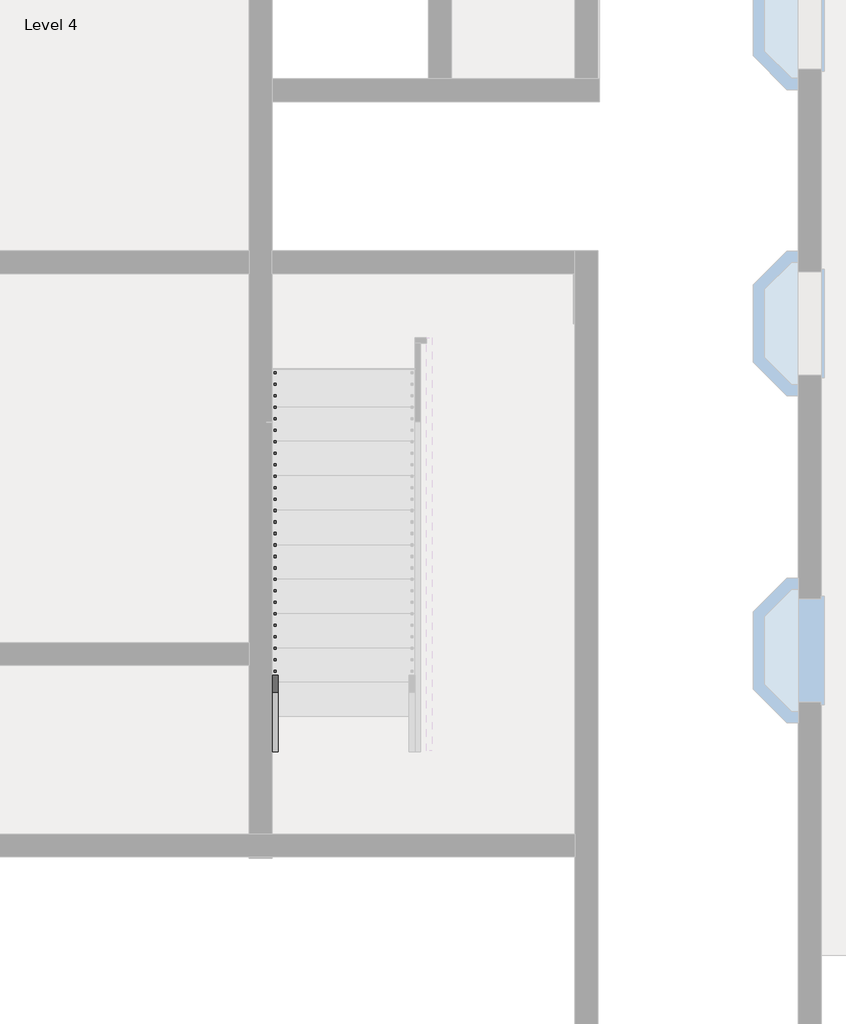
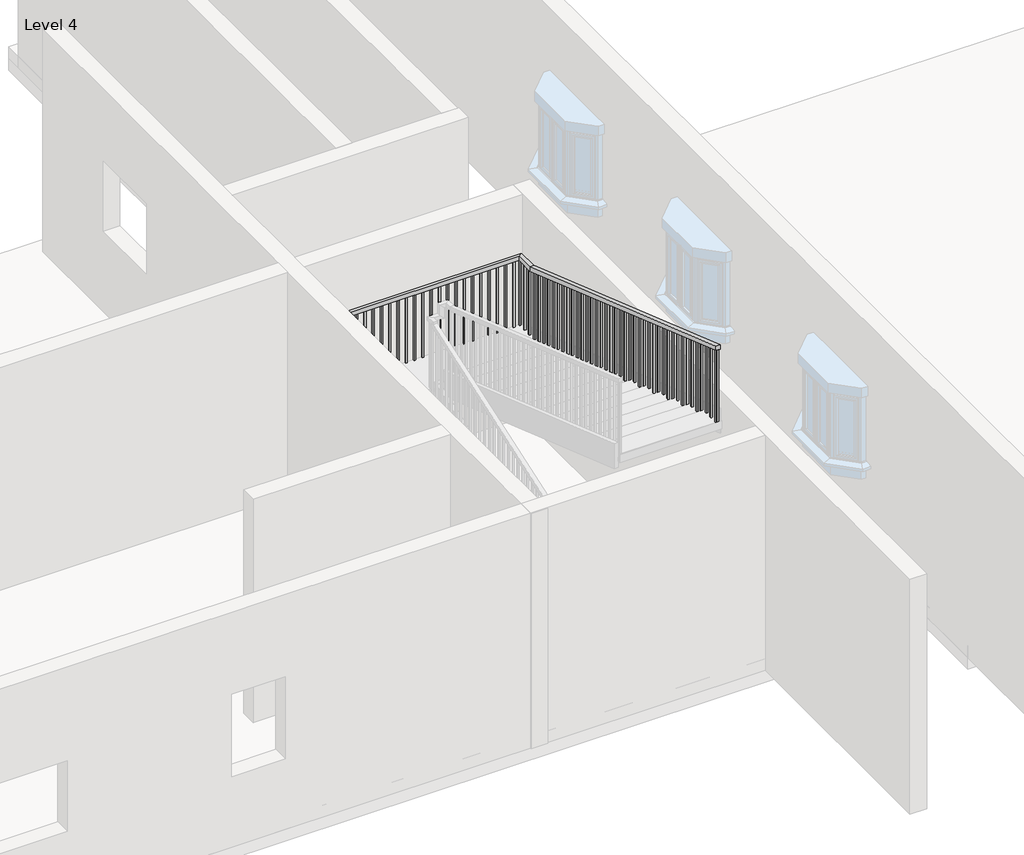
# One storey, part 8 of 14: 1 railing.
"""IFC4 building model written with IfcOpenShell, lengths in millimetres."""

from ifc_helpers import new_model, si_unit, frame, origin, place, context, project, spatial, polyline, outline, extrude, faceted_brep, element, save

model = new_model("IFC4")

# Units and contexts
model_context = context("Model", 3, world=origin())
ifc_project = project(units=[si_unit("LENGTHUNIT", "METRE", prefix="MILLI")], contexts=[model_context])

# Site, building, storey
site = spatial("IfcSite", under=ifc_project)
building = spatial("IfcBuilding", under=site)
storey = spatial("IfcBuildingStorey", under=building, Name="Level 4", Elevation=9144.0)

# Railing
placement = place(None, origin())
element("IfcRailing", 1, ObjectType="Handrail - Rectangular", at=placement, inside=storey, context=model_context, shape_type="SolidModel", body=[
    faceted_brep([(-3857.687215, -9955.5916506, 10163.9076923), (-3857.687215, -9955.5916506, 10110.1602476), (-3806.887215, -9955.5916506, 10110.1602476), (-3806.887215, -9955.5916506, 10163.9076923), (-3857.687215, -6291.6416506, 11430.0), (-3857.687215, -6283.1120276, 11379.2), (-3806.887215, -6283.1120276, 11379.2), (-3806.887215, -6291.6416506, 11430.0), (-3857.687215, -5713.7916506, 11430.0), (-3857.687215, -5713.7916506, 11379.2), (-3806.887215, -5764.5916506, 11379.2), (-3806.887215, -5764.5916506, 11430.0), (-1190.687215, -5713.7916506, 11430.0), (-1190.687215, -5713.7916506, 11379.2), (-1241.487215, -5764.5916506, 11379.2), (-1241.487215, -5764.5916506, 11430.0), (-1190.687215, -5986.8416506, 11430.0), (-1190.687215, -5995.3852679, 11379.2), (-1241.487215, -5995.3852679, 11379.2), (-1241.487215, -5986.8416506, 11430.0), (-1190.687215, -9949.2416506, 12801.6), (-1241.487215, -9949.2416506, 12801.6), (-1241.487215, -9949.2416506, 12747.842594), (-1190.687215, -9949.2416506, 12747.842594)], [[[0, 1, 2, 3]], [[1, 0, 4, 5]], [[2, 1, 5, 6]], [[3, 2, 6, 7]], [[0, 3, 7, 4]], [[5, 4, 8, 9]], [[6, 5, 9, 10]], [[7, 6, 10, 11]], [[4, 7, 11, 8]], [[9, 8, 12, 13]], [[10, 9, 13, 14]], [[11, 10, 14, 15]], [[8, 11, 15, 12]], [[13, 12, 16, 17]], [[14, 13, 17, 18]], [[15, 14, 18, 19]], [[12, 15, 19, 16]], [[20, 21, 22, 23]], [[17, 16, 20, 23]], [[18, 17, 23, 22]], [[19, 18, 22, 21]], [[16, 19, 21, 20]]]),
    extrude(outline(polyline([(-9895.2666506, 12729.1589402), (-9895.2666506, 11781.6923077), (-9914.3166506, 11781.6923077), (-9914.3166506, 12735.7531709), (-9895.2666506, 12729.1589402)])), frame((-1225.612215, 0.0, 0.0), z_axis=(1.0, 0.0, 0.0), x_axis=(0.0, 1.0, 0.0)), (0.0, 0.0, 1.0), 19.05),
    extrude(outline(polyline([(-9793.6666506, 12693.9897094), (-9793.6666506, 11781.6923077), (-9812.7166506, 11781.6923077), (-9812.7166506, 12700.5839402), (-9793.6666506, 12693.9897094)])), frame((-1225.612215, 0.0, 0.0), z_axis=(1.0, 0.0, 0.0), x_axis=(0.0, 1.0, 0.0)), (0.0, 0.0, 1.0), 19.05),
    extrude(outline(polyline([(-9692.0666506, 12658.8204786), (-9692.0666506, 11781.6923077), (-9711.1166506, 11781.6923077), (-9711.1166506, 12665.4147094), (-9692.0666506, 12658.8204786)])), frame((-1225.612215, 0.0, 0.0), z_axis=(1.0, 0.0, 0.0), x_axis=(0.0, 1.0, 0.0)), (0.0, 0.0, 1.0), 19.05),
    extrude(outline(polyline([(-9590.4666506, 12623.6512479), (-9590.4666506, 11676.1846154), (-9609.5166506, 11676.1846154), (-9609.5166506, 12630.2454786), (-9590.4666506, 12623.6512479)])), frame((-1225.612215, 0.0, 0.0), z_axis=(1.0, 0.0, 0.0), x_axis=(0.0, 1.0, 0.0)), (0.0, 0.0, 1.0), 19.05),
    extrude(outline(polyline([(-9488.8666506, 12588.4820171), (-9488.8666506, 11676.1846154), (-9507.9166506, 11676.1846154), (-9507.9166506, 12595.0762479), (-9488.8666506, 12588.4820171)])), frame((-1225.612215, 0.0, 0.0), z_axis=(1.0, 0.0, 0.0), x_axis=(0.0, 1.0, 0.0)), (0.0, 0.0, 1.0), 19.05),
    extrude(outline(polyline([(-9387.2666506, 12553.3127863), (-9387.2666506, 11676.1846154), (-9406.3166506, 11676.1846154), (-9406.3166506, 12559.9070171), (-9387.2666506, 12553.3127863)])), frame((-1225.612215, 0.0, 0.0), z_axis=(1.0, 0.0, 0.0), x_axis=(0.0, 1.0, 0.0)), (0.0, 0.0, 1.0), 19.05),
    extrude(outline(polyline([(-9285.6666506, 12518.1435556), (-9285.6666506, 11570.6769231), (-9304.7166506, 11570.6769231), (-9304.7166506, 12524.7377863), (-9285.6666506, 12518.1435556)])), frame((-1225.612215, 0.0, 0.0), z_axis=(1.0, 0.0, 0.0), x_axis=(0.0, 1.0, 0.0)), (0.0, 0.0, 1.0), 19.05),
    extrude(outline(polyline([(-9184.0666506, 12482.9743248), (-9184.0666506, 11570.6769231), (-9203.1166506, 11570.6769231), (-9203.1166506, 12489.5685556), (-9184.0666506, 12482.9743248)])), frame((-1225.612215, 0.0, 0.0), z_axis=(1.0, 0.0, 0.0), x_axis=(0.0, 1.0, 0.0)), (0.0, 0.0, 1.0), 19.05),
    extrude(outline(polyline([(-9082.4666506, 12447.805094), (-9082.4666506, 11570.6769231), (-9101.5166506, 11570.6769231), (-9101.5166506, 12454.3993248), (-9082.4666506, 12447.805094)])), frame((-1225.612215, 0.0, 0.0), z_axis=(1.0, 0.0, 0.0), x_axis=(0.0, 1.0, 0.0)), (0.0, 0.0, 1.0), 19.05),
    extrude(outline(polyline([(-8980.8666506, 12412.6358632), (-8980.8666506, 11465.1692308), (-8999.9166506, 11465.1692308), (-8999.9166506, 12419.230094), (-8980.8666506, 12412.6358632)])), frame((-1225.612215, 0.0, 0.0), z_axis=(1.0, 0.0, 0.0), x_axis=(0.0, 1.0, 0.0)), (0.0, 0.0, 1.0), 19.05),
    extrude(outline(polyline([(-8879.2666506, 12377.4666325), (-8879.2666506, 11465.1692308), (-8898.3166506, 11465.1692308), (-8898.3166506, 12384.0608632), (-8879.2666506, 12377.4666325)])), frame((-1225.612215, 0.0, 0.0), z_axis=(1.0, 0.0, 0.0), x_axis=(0.0, 1.0, 0.0)), (0.0, 0.0, 1.0), 19.05),
    extrude(outline(polyline([(-8777.6666506, 12342.2974017), (-8777.6666506, 11465.1692308), (-8796.7166506, 11465.1692308), (-8796.7166506, 12348.8916325), (-8777.6666506, 12342.2974017)])), frame((-1225.612215, 0.0, 0.0), z_axis=(1.0, 0.0, 0.0), x_axis=(0.0, 1.0, 0.0)), (0.0, 0.0, 1.0), 19.05),
    extrude(outline(polyline([(-8676.0666506, 12307.1281709), (-8676.0666506, 11359.6615385), (-8695.1166506, 11359.6615385), (-8695.1166506, 12313.7224017), (-8676.0666506, 12307.1281709)])), frame((-1225.612215, 0.0, 0.0), z_axis=(1.0, 0.0, 0.0), x_axis=(0.0, 1.0, 0.0)), (0.0, 0.0, 1.0), 19.05),
    extrude(outline(polyline([(-8574.4666506, 12271.9589402), (-8574.4666506, 11359.6615385), (-8593.5166506, 11359.6615385), (-8593.5166506, 12278.5531709), (-8574.4666506, 12271.9589402)])), frame((-1225.612215, 0.0, 0.0), z_axis=(1.0, 0.0, 0.0), x_axis=(0.0, 1.0, 0.0)), (0.0, 0.0, 1.0), 19.05),
    extrude(outline(polyline([(-8472.8666506, 12236.7897094), (-8472.8666506, 11359.6615385), (-8491.9166506, 11359.6615385), (-8491.9166506, 12243.3839402), (-8472.8666506, 12236.7897094)])), frame((-1225.612215, 0.0, 0.0), z_axis=(1.0, 0.0, 0.0), x_axis=(0.0, 1.0, 0.0)), (0.0, 0.0, 1.0), 19.05),
    extrude(outline(polyline([(-8371.2666506, 12201.6204786), (-8371.2666506, 11254.1538462), (-8390.3166506, 11254.1538462), (-8390.3166506, 12208.2147094), (-8371.2666506, 12201.6204786)])), frame((-1225.612215, 0.0, 0.0), z_axis=(1.0, 0.0, 0.0), x_axis=(0.0, 1.0, 0.0)), (0.0, 0.0, 1.0), 19.05),
    extrude(outline(polyline([(-8269.6666506, 12166.4512479), (-8269.6666506, 11254.1538462), (-8288.7166506, 11254.1538462), (-8288.7166506, 12173.0454786), (-8269.6666506, 12166.4512479)])), frame((-1225.612215, 0.0, 0.0), z_axis=(1.0, 0.0, 0.0), x_axis=(0.0, 1.0, 0.0)), (0.0, 0.0, 1.0), 19.05),
    extrude(outline(polyline([(-8168.0666506, 12131.2820171), (-8168.0666506, 11254.1538462), (-8187.1166506, 11254.1538462), (-8187.1166506, 12137.8762479), (-8168.0666506, 12131.2820171)])), frame((-1225.612215, 0.0, 0.0), z_axis=(1.0, 0.0, 0.0), x_axis=(0.0, 1.0, 0.0)), (0.0, 0.0, 1.0), 19.05),
    extrude(outline(polyline([(-8066.4666506, 12096.1127863), (-8066.4666506, 11148.6461538), (-8085.5166506, 11148.6461538), (-8085.5166506, 12102.7070171), (-8066.4666506, 12096.1127863)])), frame((-1225.612215, 0.0, 0.0), z_axis=(1.0, 0.0, 0.0), x_axis=(0.0, 1.0, 0.0)), (0.0, 0.0, 1.0), 19.05),
    extrude(outline(polyline([(-7964.8666506, 12060.9435556), (-7964.8666506, 11148.6461538), (-7983.9166506, 11148.6461538), (-7983.9166506, 12067.5377863), (-7964.8666506, 12060.9435556)])), frame((-1225.612215, 0.0, 0.0), z_axis=(1.0, 0.0, 0.0), x_axis=(0.0, 1.0, 0.0)), (0.0, 0.0, 1.0), 19.05),
    extrude(outline(polyline([(-7863.2666506, 12025.7743248), (-7863.2666506, 11148.6461538), (-7882.3166506, 11148.6461538), (-7882.3166506, 12032.3685556), (-7863.2666506, 12025.7743248)])), frame((-1225.612215, 0.0, 0.0), z_axis=(1.0, 0.0, 0.0), x_axis=(0.0, 1.0, 0.0)), (0.0, 0.0, 1.0), 19.05),
    extrude(outline(polyline([(-7761.6666506, 11990.605094), (-7761.6666506, 11043.1384615), (-7780.7166506, 11043.1384615), (-7780.7166506, 11997.1993248), (-7761.6666506, 11990.605094)])), frame((-1225.612215, 0.0, 0.0), z_axis=(1.0, 0.0, 0.0), x_axis=(0.0, 1.0, 0.0)), (0.0, 0.0, 1.0), 19.05),
    extrude(outline(polyline([(-7660.0666506, 11955.4358632), (-7660.0666506, 11043.1384615), (-7679.1166506, 11043.1384615), (-7679.1166506, 11962.030094), (-7660.0666506, 11955.4358632)])), frame((-1225.612215, 0.0, 0.0), z_axis=(1.0, 0.0, 0.0), x_axis=(0.0, 1.0, 0.0)), (0.0, 0.0, 1.0), 19.05),
    extrude(outline(polyline([(-7558.4666506, 11920.2666325), (-7558.4666506, 11043.1384615), (-7577.5166506, 11043.1384615), (-7577.5166506, 11926.8608632), (-7558.4666506, 11920.2666325)])), frame((-1225.612215, 0.0, 0.0), z_axis=(1.0, 0.0, 0.0), x_axis=(0.0, 1.0, 0.0)), (0.0, 0.0, 1.0), 19.05),
    extrude(outline(polyline([(-7456.8666506, 11885.0974017), (-7456.8666506, 10937.6307692), (-7475.9166506, 10937.6307692), (-7475.9166506, 11891.6916325), (-7456.8666506, 11885.0974017)])), frame((-1225.612215, 0.0, 0.0), z_axis=(1.0, 0.0, 0.0), x_axis=(0.0, 1.0, 0.0)), (0.0, 0.0, 1.0), 19.05),
    extrude(outline(polyline([(-7355.2666506, 11849.9281709), (-7355.2666506, 10937.6307692), (-7374.3166506, 10937.6307692), (-7374.3166506, 11856.5224017), (-7355.2666506, 11849.9281709)])), frame((-1225.612215, 0.0, 0.0), z_axis=(1.0, 0.0, 0.0), x_axis=(0.0, 1.0, 0.0)), (0.0, 0.0, 1.0), 19.05),
    extrude(outline(polyline([(-7253.6666506, 11814.7589402), (-7253.6666506, 10937.6307692), (-7272.7166506, 10937.6307692), (-7272.7166506, 11821.3531709), (-7253.6666506, 11814.7589402)])), frame((-1225.612215, 0.0, 0.0), z_axis=(1.0, 0.0, 0.0), x_axis=(0.0, 1.0, 0.0)), (0.0, 0.0, 1.0), 19.05),
    extrude(outline(polyline([(-7152.0666506, 11779.5897094), (-7152.0666506, 10832.1230769), (-7171.1166506, 10832.1230769), (-7171.1166506, 11786.1839402), (-7152.0666506, 11779.5897094)])), frame((-1225.612215, 0.0, 0.0), z_axis=(1.0, 0.0, 0.0), x_axis=(0.0, 1.0, 0.0)), (0.0, 0.0, 1.0), 19.05),
    extrude(outline(polyline([(-7050.4666506, 11744.4204786), (-7050.4666506, 10832.1230769), (-7069.5166506, 10832.1230769), (-7069.5166506, 11751.0147094), (-7050.4666506, 11744.4204786)])), frame((-1225.612215, 0.0, 0.0), z_axis=(1.0, 0.0, 0.0), x_axis=(0.0, 1.0, 0.0)), (0.0, 0.0, 1.0), 19.05),
    extrude(outline(polyline([(-6948.8666506, 11709.2512479), (-6948.8666506, 10832.1230769), (-6967.9166506, 10832.1230769), (-6967.9166506, 11715.8454786), (-6948.8666506, 11709.2512479)])), frame((-1225.612215, 0.0, 0.0), z_axis=(1.0, 0.0, 0.0), x_axis=(0.0, 1.0, 0.0)), (0.0, 0.0, 1.0), 19.05),
    extrude(outline(polyline([(-6847.2666506, 11674.0820171), (-6847.2666506, 10726.6153846), (-6866.3166506, 10726.6153846), (-6866.3166506, 11680.6762479), (-6847.2666506, 11674.0820171)])), frame((-1225.612215, 0.0, 0.0), z_axis=(1.0, 0.0, 0.0), x_axis=(0.0, 1.0, 0.0)), (0.0, 0.0, 1.0), 19.05),
    extrude(outline(polyline([(-6745.6666506, 11638.9127863), (-6745.6666506, 10726.6153846), (-6764.7166506, 10726.6153846), (-6764.7166506, 11645.5070171), (-6745.6666506, 11638.9127863)])), frame((-1225.612215, 0.0, 0.0), z_axis=(1.0, 0.0, 0.0), x_axis=(0.0, 1.0, 0.0)), (0.0, 0.0, 1.0), 19.05),
    extrude(outline(polyline([(-6644.0666506, 11603.7435556), (-6644.0666506, 10726.6153846), (-6663.1166506, 10726.6153846), (-6663.1166506, 11610.3377863), (-6644.0666506, 11603.7435556)])), frame((-1225.612215, 0.0, 0.0), z_axis=(1.0, 0.0, 0.0), x_axis=(0.0, 1.0, 0.0)), (0.0, 0.0, 1.0), 19.05),
    extrude(outline(polyline([(-6542.4666506, 11568.5743248), (-6542.4666506, 10621.1076923), (-6561.5166506, 10621.1076923), (-6561.5166506, 11575.1685556), (-6542.4666506, 11568.5743248)])), frame((-1225.612215, 0.0, 0.0), z_axis=(1.0, 0.0, 0.0), x_axis=(0.0, 1.0, 0.0)), (0.0, 0.0, 1.0), 19.05),
    extrude(outline(polyline([(-6440.8666506, 11533.405094), (-6440.8666506, 10621.1076923), (-6459.9166506, 10621.1076923), (-6459.9166506, 11539.9993248), (-6440.8666506, 11533.405094)])), frame((-1225.612215, 0.0, 0.0), z_axis=(1.0, 0.0, 0.0), x_axis=(0.0, 1.0, 0.0)), (0.0, 0.0, 1.0), 19.05),
    extrude(outline(polyline([(-6339.2666506, 11498.2358632), (-6339.2666506, 10621.1076923), (-6358.3166506, 10621.1076923), (-6358.3166506, 11504.830094), (-6339.2666506, 11498.2358632)])), frame((-1225.612215, 0.0, 0.0), z_axis=(1.0, 0.0, 0.0), x_axis=(0.0, 1.0, 0.0)), (0.0, 0.0, 1.0), 19.05),
    extrude(outline(polyline([(-6237.6666506, 11463.0666325), (-6237.6666506, 10515.6), (-6256.7166506, 10515.6), (-6256.7166506, 11469.6608632), (-6237.6666506, 11463.0666325)])), frame((-1225.612215, 0.0, 0.0), z_axis=(1.0, 0.0, 0.0), x_axis=(0.0, 1.0, 0.0)), (0.0, 0.0, 1.0), 19.05),
    extrude(outline(polyline([(-6136.0666506, 11427.8974017), (-6136.0666506, 10515.6), (-6155.1166506, 10515.6), (-6155.1166506, 11434.4916325), (-6136.0666506, 11427.8974017)])), frame((-1225.612215, 0.0, 0.0), z_axis=(1.0, 0.0, 0.0), x_axis=(0.0, 1.0, 0.0)), (0.0, 0.0, 1.0), 19.05),
    extrude(outline(polyline([(-6034.4666506, 11392.7281709), (-6034.4666506, 10515.6), (-6053.5166506, 10515.6), (-6053.5166506, 11399.3224017), (-6034.4666506, 11392.7281709)])), frame((-1225.612215, 0.0, 0.0), z_axis=(1.0, 0.0, 0.0), x_axis=(0.0, 1.0, 0.0)), (0.0, 0.0, 1.0), 19.05),
    extrude(outline(polyline([(-1206.562215, -5932.8666506), (-1206.562215, -5951.9166506), (-1225.612215, -5951.9166506), (-1225.612215, -5932.8666506), (-1206.562215, -5932.8666506)])), frame((0.0, 0.0, 10515.6), z_axis=(0.0, 0.0, 1.0), x_axis=(1.0, 0.0, 0.0)), (0.0, 0.0, 1.0), 863.6),
    extrude(outline(polyline([(-1206.562215, -5831.2666506), (-1206.562215, -5850.3166506), (-1225.612215, -5850.3166506), (-1225.612215, -5831.2666506), (-1206.562215, -5831.2666506)])), frame((0.0, 0.0, 10515.6), z_axis=(0.0, 0.0, 1.0), x_axis=(1.0, 0.0, 0.0)), (0.0, 0.0, 1.0), 863.6),
    extrude(outline(polyline([(-1301.812215, -5729.6666506), (-1282.762215, -5729.6666506), (-1282.762215, -5748.7166506), (-1301.812215, -5748.7166506), (-1301.812215, -5729.6666506)])), frame((0.0, 0.0, 10515.6), z_axis=(0.0, 0.0, 1.0), x_axis=(1.0, 0.0, 0.0)), (0.0, 0.0, 1.0), 863.6),
    extrude(outline(polyline([(-1403.412215, -5729.6666506), (-1384.362215, -5729.6666506), (-1384.362215, -5748.7166506), (-1403.412215, -5748.7166506), (-1403.412215, -5729.6666506)])), frame((0.0, 0.0, 10515.6), z_axis=(0.0, 0.0, 1.0), x_axis=(1.0, 0.0, 0.0)), (0.0, 0.0, 1.0), 863.6),
    extrude(outline(polyline([(-1505.012215, -5729.6666506), (-1485.962215, -5729.6666506), (-1485.962215, -5748.7166506), (-1505.012215, -5748.7166506), (-1505.012215, -5729.6666506)])), frame((0.0, 0.0, 10515.6), z_axis=(0.0, 0.0, 1.0), x_axis=(1.0, 0.0, 0.0)), (0.0, 0.0, 1.0), 863.6),
    extrude(outline(polyline([(-1606.612215, -5729.6666506), (-1587.562215, -5729.6666506), (-1587.562215, -5748.7166506), (-1606.612215, -5748.7166506), (-1606.612215, -5729.6666506)])), frame((0.0, 0.0, 10515.6), z_axis=(0.0, 0.0, 1.0), x_axis=(1.0, 0.0, 0.0)), (0.0, 0.0, 1.0), 863.6),
    extrude(outline(polyline([(-1708.212215, -5729.6666506), (-1689.162215, -5729.6666506), (-1689.162215, -5748.7166506), (-1708.212215, -5748.7166506), (-1708.212215, -5729.6666506)])), frame((0.0, 0.0, 10515.6), z_axis=(0.0, 0.0, 1.0), x_axis=(1.0, 0.0, 0.0)), (0.0, 0.0, 1.0), 863.6),
    extrude(outline(polyline([(-1809.812215, -5729.6666506), (-1790.762215, -5729.6666506), (-1790.762215, -5748.7166506), (-1809.812215, -5748.7166506), (-1809.812215, -5729.6666506)])), frame((0.0, 0.0, 10515.6), z_axis=(0.0, 0.0, 1.0), x_axis=(1.0, 0.0, 0.0)), (0.0, 0.0, 1.0), 863.6),
    extrude(outline(polyline([(-1911.412215, -5729.6666506), (-1892.362215, -5729.6666506), (-1892.362215, -5748.7166506), (-1911.412215, -5748.7166506), (-1911.412215, -5729.6666506)])), frame((0.0, 0.0, 10515.6), z_axis=(0.0, 0.0, 1.0), x_axis=(1.0, 0.0, 0.0)), (0.0, 0.0, 1.0), 863.6),
    extrude(outline(polyline([(-2013.012215, -5729.6666506), (-1993.962215, -5729.6666506), (-1993.962215, -5748.7166506), (-2013.012215, -5748.7166506), (-2013.012215, -5729.6666506)])), frame((0.0, 0.0, 10515.6), z_axis=(0.0, 0.0, 1.0), x_axis=(1.0, 0.0, 0.0)), (0.0, 0.0, 1.0), 863.6),
    extrude(outline(polyline([(-2114.612215, -5729.6666506), (-2095.562215, -5729.6666506), (-2095.562215, -5748.7166506), (-2114.612215, -5748.7166506), (-2114.612215, -5729.6666506)])), frame((0.0, 0.0, 10515.6), z_axis=(0.0, 0.0, 1.0), x_axis=(1.0, 0.0, 0.0)), (0.0, 0.0, 1.0), 863.6),
    extrude(outline(polyline([(-2216.212215, -5729.6666506), (-2197.162215, -5729.6666506), (-2197.162215, -5748.7166506), (-2216.212215, -5748.7166506), (-2216.212215, -5729.6666506)])), frame((0.0, 0.0, 10515.6), z_axis=(0.0, 0.0, 1.0), x_axis=(1.0, 0.0, 0.0)), (0.0, 0.0, 1.0), 863.6),
    extrude(outline(polyline([(-2317.812215, -5729.6666506), (-2298.762215, -5729.6666506), (-2298.762215, -5748.7166506), (-2317.812215, -5748.7166506), (-2317.812215, -5729.6666506)])), frame((0.0, 0.0, 10515.6), z_axis=(0.0, 0.0, 1.0), x_axis=(1.0, 0.0, 0.0)), (0.0, 0.0, 1.0), 863.6),
    extrude(outline(polyline([(-2419.412215, -5729.6666506), (-2400.362215, -5729.6666506), (-2400.362215, -5748.7166506), (-2419.412215, -5748.7166506), (-2419.412215, -5729.6666506)])), frame((0.0, 0.0, 10515.6), z_axis=(0.0, 0.0, 1.0), x_axis=(1.0, 0.0, 0.0)), (0.0, 0.0, 1.0), 863.6),
    extrude(outline(polyline([(-2521.012215, -5729.6666506), (-2501.962215, -5729.6666506), (-2501.962215, -5748.7166506), (-2521.012215, -5748.7166506), (-2521.012215, -5729.6666506)])), frame((0.0, 0.0, 10515.6), z_axis=(0.0, 0.0, 1.0), x_axis=(1.0, 0.0, 0.0)), (0.0, 0.0, 1.0), 863.6),
    extrude(outline(polyline([(-2622.612215, -5729.6666506), (-2603.562215, -5729.6666506), (-2603.562215, -5748.7166506), (-2622.612215, -5748.7166506), (-2622.612215, -5729.6666506)])), frame((0.0, 0.0, 10515.6), z_axis=(0.0, 0.0, 1.0), x_axis=(1.0, 0.0, 0.0)), (0.0, 0.0, 1.0), 863.6),
    extrude(outline(polyline([(-2724.212215, -5729.6666506), (-2705.162215, -5729.6666506), (-2705.162215, -5748.7166506), (-2724.212215, -5748.7166506), (-2724.212215, -5729.6666506)])), frame((0.0, 0.0, 10515.6), z_axis=(0.0, 0.0, 1.0), x_axis=(1.0, 0.0, 0.0)), (0.0, 0.0, 1.0), 863.6),
    extrude(outline(polyline([(-2825.812215, -5729.6666506), (-2806.762215, -5729.6666506), (-2806.762215, -5748.7166506), (-2825.812215, -5748.7166506), (-2825.812215, -5729.6666506)])), frame((0.0, 0.0, 10515.6), z_axis=(0.0, 0.0, 1.0), x_axis=(1.0, 0.0, 0.0)), (0.0, 0.0, 1.0), 863.6),
    extrude(outline(polyline([(-2927.412215, -5729.6666506), (-2908.362215, -5729.6666506), (-2908.362215, -5748.7166506), (-2927.412215, -5748.7166506), (-2927.412215, -5729.6666506)])), frame((0.0, 0.0, 10515.6), z_axis=(0.0, 0.0, 1.0), x_axis=(1.0, 0.0, 0.0)), (0.0, 0.0, 1.0), 863.6),
    extrude(outline(polyline([(-3029.012215, -5729.6666506), (-3009.962215, -5729.6666506), (-3009.962215, -5748.7166506), (-3029.012215, -5748.7166506), (-3029.012215, -5729.6666506)])), frame((0.0, 0.0, 10515.6), z_axis=(0.0, 0.0, 1.0), x_axis=(1.0, 0.0, 0.0)), (0.0, 0.0, 1.0), 863.6),
    extrude(outline(polyline([(-3130.612215, -5729.6666506), (-3111.562215, -5729.6666506), (-3111.562215, -5748.7166506), (-3130.612215, -5748.7166506), (-3130.612215, -5729.6666506)])), frame((0.0, 0.0, 10515.6), z_axis=(0.0, 0.0, 1.0), x_axis=(1.0, 0.0, 0.0)), (0.0, 0.0, 1.0), 863.6),
    extrude(outline(polyline([(-3232.212215, -5729.6666506), (-3213.162215, -5729.6666506), (-3213.162215, -5748.7166506), (-3232.212215, -5748.7166506), (-3232.212215, -5729.6666506)])), frame((0.0, 0.0, 10515.6), z_axis=(0.0, 0.0, 1.0), x_axis=(1.0, 0.0, 0.0)), (0.0, 0.0, 1.0), 863.6),
    extrude(outline(polyline([(-3333.812215, -5729.6666506), (-3314.762215, -5729.6666506), (-3314.762215, -5748.7166506), (-3333.812215, -5748.7166506), (-3333.812215, -5729.6666506)])), frame((0.0, 0.0, 10515.6), z_axis=(0.0, 0.0, 1.0), x_axis=(1.0, 0.0, 0.0)), (0.0, 0.0, 1.0), 863.6),
    extrude(outline(polyline([(-3435.412215, -5729.6666506), (-3416.362215, -5729.6666506), (-3416.362215, -5748.7166506), (-3435.412215, -5748.7166506), (-3435.412215, -5729.6666506)])), frame((0.0, 0.0, 10515.6), z_axis=(0.0, 0.0, 1.0), x_axis=(1.0, 0.0, 0.0)), (0.0, 0.0, 1.0), 863.6),
    extrude(outline(polyline([(-3537.012215, -5729.6666506), (-3517.962215, -5729.6666506), (-3517.962215, -5748.7166506), (-3537.012215, -5748.7166506), (-3537.012215, -5729.6666506)])), frame((0.0, 0.0, 10515.6), z_axis=(0.0, 0.0, 1.0), x_axis=(1.0, 0.0, 0.0)), (0.0, 0.0, 1.0), 863.6),
    extrude(outline(polyline([(-3638.612215, -5729.6666506), (-3619.562215, -5729.6666506), (-3619.562215, -5748.7166506), (-3638.612215, -5748.7166506), (-3638.612215, -5729.6666506)])), frame((0.0, 0.0, 10515.6), z_axis=(0.0, 0.0, 1.0), x_axis=(1.0, 0.0, 0.0)), (0.0, 0.0, 1.0), 863.6),
    extrude(outline(polyline([(-3740.212215, -5729.6666506), (-3721.162215, -5729.6666506), (-3721.162215, -5748.7166506), (-3740.212215, -5748.7166506), (-3740.212215, -5729.6666506)])), frame((0.0, 0.0, 10515.6), z_axis=(0.0, 0.0, 1.0), x_axis=(1.0, 0.0, 0.0)), (0.0, 0.0, 1.0), 863.6),
    extrude(outline(polyline([(-3841.812215, -5799.5166506), (-3841.812215, -5780.4666506), (-3822.762215, -5780.4666506), (-3822.762215, -5799.5166506), (-3841.812215, -5799.5166506)])), frame((0.0, 0.0, 10515.6), z_axis=(0.0, 0.0, 1.0), x_axis=(1.0, 0.0, 0.0)), (0.0, 0.0, 1.0), 863.6),
    extrude(outline(polyline([(-3841.812215, -5901.1166506), (-3841.812215, -5882.0666506), (-3822.762215, -5882.0666506), (-3822.762215, -5901.1166506), (-3841.812215, -5901.1166506)])), frame((0.0, 0.0, 10515.6), z_axis=(0.0, 0.0, 1.0), x_axis=(1.0, 0.0, 0.0)), (0.0, 0.0, 1.0), 863.6),
    extrude(outline(polyline([(-3841.812215, -6002.7166506), (-3841.812215, -5983.6666506), (-3822.762215, -5983.6666506), (-3822.762215, -6002.7166506), (-3841.812215, -6002.7166506)])), frame((0.0, 0.0, 10515.6), z_axis=(0.0, 0.0, 1.0), x_axis=(1.0, 0.0, 0.0)), (0.0, 0.0, 1.0), 863.6),
    extrude(outline(polyline([(-3841.812215, -6104.3166506), (-3841.812215, -6085.2666506), (-3822.762215, -6085.2666506), (-3822.762215, -6104.3166506), (-3841.812215, -6104.3166506)])), frame((0.0, 0.0, 10515.6), z_axis=(0.0, 0.0, 1.0), x_axis=(1.0, 0.0, 0.0)), (0.0, 0.0, 1.0), 863.6),
    extrude(outline(polyline([(-3841.812215, -6205.9166506), (-3841.812215, -6186.8666506), (-3822.762215, -6186.8666506), (-3822.762215, -6205.9166506), (-3841.812215, -6205.9166506)])), frame((0.0, 0.0, 10515.6), z_axis=(0.0, 0.0, 1.0), x_axis=(1.0, 0.0, 0.0)), (0.0, 0.0, 1.0), 863.6),
    extrude(outline(polyline([(-6288.4666506, 11377.349689), (-6288.4666506, 10410.0923077), (-6307.5166506, 10410.0923077), (-6307.5166506, 11370.7668867), (-6288.4666506, 11377.349689)])), frame((-3841.812215, 0.0, 0.0), z_axis=(1.0, 0.0, 0.0), x_axis=(0.0, 1.0, 0.0)), (0.0, 0.0, 1.0), 19.05),
    extrude(outline(polyline([(-6390.0666506, 11342.2414101), (-6390.0666506, 10410.0923077), (-6409.1166506, 10410.0923077), (-6409.1166506, 11335.6586078), (-6390.0666506, 11342.2414101)])), frame((-3841.812215, 0.0, 0.0), z_axis=(1.0, 0.0, 0.0), x_axis=(0.0, 1.0, 0.0)), (0.0, 0.0, 1.0), 19.05),
    extrude(outline(polyline([(-6491.6666506, 11307.1331312), (-6491.6666506, 10410.0923077), (-6510.7166506, 10410.0923077), (-6510.7166506, 11300.5503289), (-6491.6666506, 11307.1331312)])), frame((-3841.812215, 0.0, 0.0), z_axis=(1.0, 0.0, 0.0), x_axis=(0.0, 1.0, 0.0)), (0.0, 0.0, 1.0), 19.05),
    extrude(outline(polyline([(-6593.2666506, 11272.0248523), (-6593.2666506, 10304.5846154), (-6612.3166506, 10304.5846154), (-6612.3166506, 11265.44205), (-6593.2666506, 11272.0248523)])), frame((-3841.812215, 0.0, 0.0), z_axis=(1.0, 0.0, 0.0), x_axis=(0.0, 1.0, 0.0)), (0.0, 0.0, 1.0), 19.05),
    extrude(outline(polyline([(-6694.8666506, 11236.9165734), (-6694.8666506, 10304.5846154), (-6713.9166506, 10304.5846154), (-6713.9166506, 11230.3337711), (-6694.8666506, 11236.9165734)])), frame((-3841.812215, 0.0, 0.0), z_axis=(1.0, 0.0, 0.0), x_axis=(0.0, 1.0, 0.0)), (0.0, 0.0, 1.0), 19.05),
    extrude(outline(polyline([(-6796.4666506, 11201.8082945), (-6796.4666506, 10304.5846154), (-6815.5166506, 10304.5846154), (-6815.5166506, 11195.2254922), (-6796.4666506, 11201.8082945)])), frame((-3841.812215, 0.0, 0.0), z_axis=(1.0, 0.0, 0.0), x_axis=(0.0, 1.0, 0.0)), (0.0, 0.0, 1.0), 19.05),
    extrude(outline(polyline([(-6898.0666506, 11166.7000156), (-6898.0666506, 10199.0769231), (-6917.1166506, 10199.0769231), (-6917.1166506, 11160.1172133), (-6898.0666506, 11166.7000156)])), frame((-3841.812215, 0.0, 0.0), z_axis=(1.0, 0.0, 0.0), x_axis=(0.0, 1.0, 0.0)), (0.0, 0.0, 1.0), 19.05),
    extrude(outline(polyline([(-6999.6666506, 11131.5917367), (-6999.6666506, 10199.0769231), (-7018.7166506, 10199.0769231), (-7018.7166506, 11125.0089344), (-6999.6666506, 11131.5917367)])), frame((-3841.812215, 0.0, 0.0), z_axis=(1.0, 0.0, 0.0), x_axis=(0.0, 1.0, 0.0)), (0.0, 0.0, 1.0), 19.05),
    extrude(outline(polyline([(-7101.2666506, 11096.4834578), (-7101.2666506, 10199.0769231), (-7120.3166506, 10199.0769231), (-7120.3166506, 11089.9006556), (-7101.2666506, 11096.4834578)])), frame((-3841.812215, 0.0, 0.0), z_axis=(1.0, 0.0, 0.0), x_axis=(0.0, 1.0, 0.0)), (0.0, 0.0, 1.0), 19.05),
    extrude(outline(polyline([(-7202.8666506, 11061.375179), (-7202.8666506, 10093.5692308), (-7221.9166506, 10093.5692308), (-7221.9166506, 11054.7923767), (-7202.8666506, 11061.375179)])), frame((-3841.812215, 0.0, 0.0), z_axis=(1.0, 0.0, 0.0), x_axis=(0.0, 1.0, 0.0)), (0.0, 0.0, 1.0), 19.05),
    extrude(outline(polyline([(-7304.4666506, 11026.2669001), (-7304.4666506, 10093.5692308), (-7323.5166506, 10093.5692308), (-7323.5166506, 11019.6840978), (-7304.4666506, 11026.2669001)])), frame((-3841.812215, 0.0, 0.0), z_axis=(1.0, 0.0, 0.0), x_axis=(0.0, 1.0, 0.0)), (0.0, 0.0, 1.0), 19.05),
    extrude(outline(polyline([(-7406.0666506, 10991.1586212), (-7406.0666506, 10093.5692308), (-7425.1166506, 10093.5692308), (-7425.1166506, 10984.5758189), (-7406.0666506, 10991.1586212)])), frame((-3841.812215, 0.0, 0.0), z_axis=(1.0, 0.0, 0.0), x_axis=(0.0, 1.0, 0.0)), (0.0, 0.0, 1.0), 19.05),
    extrude(outline(polyline([(-7507.6666506, 10956.0503423), (-7507.6666506, 9988.0615385), (-7526.7166506, 9988.0615385), (-7526.7166506, 10949.46754), (-7507.6666506, 10956.0503423)])), frame((-3841.812215, 0.0, 0.0), z_axis=(1.0, 0.0, 0.0), x_axis=(0.0, 1.0, 0.0)), (0.0, 0.0, 1.0), 19.05),
    extrude(outline(polyline([(-7609.2666506, 10920.9420634), (-7609.2666506, 9988.0615385), (-7628.3166506, 9988.0615385), (-7628.3166506, 10914.3592611), (-7609.2666506, 10920.9420634)])), frame((-3841.812215, 0.0, 0.0), z_axis=(1.0, 0.0, 0.0), x_axis=(0.0, 1.0, 0.0)), (0.0, 0.0, 1.0), 19.05),
    extrude(outline(polyline([(-7710.8666506, 10885.8337845), (-7710.8666506, 9988.0615385), (-7729.9166506, 9988.0615385), (-7729.9166506, 10879.2509822), (-7710.8666506, 10885.8337845)])), frame((-3841.812215, 0.0, 0.0), z_axis=(1.0, 0.0, 0.0), x_axis=(0.0, 1.0, 0.0)), (0.0, 0.0, 1.0), 19.05),
    extrude(outline(polyline([(-7812.4666506, 10850.7255056), (-7812.4666506, 9882.5538462), (-7831.5166506, 9882.5538462), (-7831.5166506, 10844.1427033), (-7812.4666506, 10850.7255056)])), frame((-3841.812215, 0.0, 0.0), z_axis=(1.0, 0.0, 0.0), x_axis=(0.0, 1.0, 0.0)), (0.0, 0.0, 1.0), 19.05),
    extrude(outline(polyline([(-7914.0666506, 10815.6172267), (-7914.0666506, 9882.5538462), (-7933.1166506, 9882.5538462), (-7933.1166506, 10809.0344244), (-7914.0666506, 10815.6172267)])), frame((-3841.812215, 0.0, 0.0), z_axis=(1.0, 0.0, 0.0), x_axis=(0.0, 1.0, 0.0)), (0.0, 0.0, 1.0), 19.05),
    extrude(outline(polyline([(-8015.6666506, 10780.5089478), (-8015.6666506, 9882.5538462), (-8034.7166506, 9882.5538462), (-8034.7166506, 10773.9261455), (-8015.6666506, 10780.5089478)])), frame((-3841.812215, 0.0, 0.0), z_axis=(1.0, 0.0, 0.0), x_axis=(0.0, 1.0, 0.0)), (0.0, 0.0, 1.0), 19.05),
    extrude(outline(polyline([(-8117.2666506, 10745.4006689), (-8117.2666506, 9777.0461538), (-8136.3166506, 9777.0461538), (-8136.3166506, 10738.8178666), (-8117.2666506, 10745.4006689)])), frame((-3841.812215, 0.0, 0.0), z_axis=(1.0, 0.0, 0.0), x_axis=(0.0, 1.0, 0.0)), (0.0, 0.0, 1.0), 19.05),
    extrude(outline(polyline([(-8218.8666506, 10710.29239), (-8218.8666506, 9777.0461538), (-8237.9166506, 9777.0461538), (-8237.9166506, 10703.7095877), (-8218.8666506, 10710.29239)])), frame((-3841.812215, 0.0, 0.0), z_axis=(1.0, 0.0, 0.0), x_axis=(0.0, 1.0, 0.0)), (0.0, 0.0, 1.0), 19.05),
    extrude(outline(polyline([(-8320.4666506, 10675.1841111), (-8320.4666506, 9777.0461538), (-8339.5166506, 9777.0461538), (-8339.5166506, 10668.6013088), (-8320.4666506, 10675.1841111)])), frame((-3841.812215, 0.0, 0.0), z_axis=(1.0, 0.0, 0.0), x_axis=(0.0, 1.0, 0.0)), (0.0, 0.0, 1.0), 19.05),
    extrude(outline(polyline([(-8422.0666506, 10640.0758322), (-8422.0666506, 9671.5384615), (-8441.1166506, 9671.5384615), (-8441.1166506, 10633.4930299), (-8422.0666506, 10640.0758322)])), frame((-3841.812215, 0.0, 0.0), z_axis=(1.0, 0.0, 0.0), x_axis=(0.0, 1.0, 0.0)), (0.0, 0.0, 1.0), 19.05),
    extrude(outline(polyline([(-8523.6666506, 10604.9675533), (-8523.6666506, 9671.5384615), (-8542.7166506, 9671.5384615), (-8542.7166506, 10598.384751), (-8523.6666506, 10604.9675533)])), frame((-3841.812215, 0.0, 0.0), z_axis=(1.0, 0.0, 0.0), x_axis=(0.0, 1.0, 0.0)), (0.0, 0.0, 1.0), 19.05),
    extrude(outline(polyline([(-8625.2666506, 10569.8592744), (-8625.2666506, 9671.5384615), (-8644.3166506, 9671.5384615), (-8644.3166506, 10563.2764721), (-8625.2666506, 10569.8592744)])), frame((-3841.812215, 0.0, 0.0), z_axis=(1.0, 0.0, 0.0), x_axis=(0.0, 1.0, 0.0)), (0.0, 0.0, 1.0), 19.05),
    extrude(outline(polyline([(-8726.8666506, 10534.7509955), (-8726.8666506, 9566.0307692), (-8745.9166506, 9566.0307692), (-8745.9166506, 10528.1681932), (-8726.8666506, 10534.7509955)])), frame((-3841.812215, 0.0, 0.0), z_axis=(1.0, 0.0, 0.0), x_axis=(0.0, 1.0, 0.0)), (0.0, 0.0, 1.0), 19.05),
    extrude(outline(polyline([(-8828.4666506, 10499.6427166), (-8828.4666506, 9566.0307692), (-8847.5166506, 9566.0307692), (-8847.5166506, 10493.0599143), (-8828.4666506, 10499.6427166)])), frame((-3841.812215, 0.0, 0.0), z_axis=(1.0, 0.0, 0.0), x_axis=(0.0, 1.0, 0.0)), (0.0, 0.0, 1.0), 19.05),
    extrude(outline(polyline([(-8930.0666506, 10464.5344377), (-8930.0666506, 9566.0307692), (-8949.1166506, 9566.0307692), (-8949.1166506, 10457.9516354), (-8930.0666506, 10464.5344377)])), frame((-3841.812215, 0.0, 0.0), z_axis=(1.0, 0.0, 0.0), x_axis=(0.0, 1.0, 0.0)), (0.0, 0.0, 1.0), 19.05),
    extrude(outline(polyline([(-9031.6666506, 10429.4261588), (-9031.6666506, 9460.5230769), (-9050.7166506, 9460.5230769), (-9050.7166506, 10422.8433565), (-9031.6666506, 10429.4261588)])), frame((-3841.812215, 0.0, 0.0), z_axis=(1.0, 0.0, 0.0), x_axis=(0.0, 1.0, 0.0)), (0.0, 0.0, 1.0), 19.05),
    extrude(outline(polyline([(-9133.2666506, 10394.3178799), (-9133.2666506, 9460.5230769), (-9152.3166506, 9460.5230769), (-9152.3166506, 10387.7350776), (-9133.2666506, 10394.3178799)])), frame((-3841.812215, 0.0, 0.0), z_axis=(1.0, 0.0, 0.0), x_axis=(0.0, 1.0, 0.0)), (0.0, 0.0, 1.0), 19.05),
    extrude(outline(polyline([(-9234.8666506, 10359.209601), (-9234.8666506, 9460.5230769), (-9253.9166506, 9460.5230769), (-9253.9166506, 10352.6267987), (-9234.8666506, 10359.209601)])), frame((-3841.812215, 0.0, 0.0), z_axis=(1.0, 0.0, 0.0), x_axis=(0.0, 1.0, 0.0)), (0.0, 0.0, 1.0), 19.05),
    extrude(outline(polyline([(-9336.4666506, 10324.1013221), (-9336.4666506, 9355.0153846), (-9355.5166506, 9355.0153846), (-9355.5166506, 10317.5185198), (-9336.4666506, 10324.1013221)])), frame((-3841.812215, 0.0, 0.0), z_axis=(1.0, 0.0, 0.0), x_axis=(0.0, 1.0, 0.0)), (0.0, 0.0, 1.0), 19.05),
    extrude(outline(polyline([(-9438.0666506, 10288.9930432), (-9438.0666506, 9355.0153846), (-9457.1166506, 9355.0153846), (-9457.1166506, 10282.4102409), (-9438.0666506, 10288.9930432)])), frame((-3841.812215, 0.0, 0.0), z_axis=(1.0, 0.0, 0.0), x_axis=(0.0, 1.0, 0.0)), (0.0, 0.0, 1.0), 19.05),
    extrude(outline(polyline([(-9539.6666506, 10253.8847643), (-9539.6666506, 9355.0153846), (-9558.7166506, 9355.0153846), (-9558.7166506, 10247.301962), (-9539.6666506, 10253.8847643)])), frame((-3841.812215, 0.0, 0.0), z_axis=(1.0, 0.0, 0.0), x_axis=(0.0, 1.0, 0.0)), (0.0, 0.0, 1.0), 19.05),
    extrude(outline(polyline([(-9641.2666506, 10218.7764854), (-9641.2666506, 9249.5076923), (-9660.3166506, 9249.5076923), (-9660.3166506, 10212.1936831), (-9641.2666506, 10218.7764854)])), frame((-3841.812215, 0.0, 0.0), z_axis=(1.0, 0.0, 0.0), x_axis=(0.0, 1.0, 0.0)), (0.0, 0.0, 1.0), 19.05),
    extrude(outline(polyline([(-9742.8666506, 10183.6682065), (-9742.8666506, 9249.5076923), (-9761.9166506, 9249.5076923), (-9761.9166506, 10177.0854043), (-9742.8666506, 10183.6682065)])), frame((-3841.812215, 0.0, 0.0), z_axis=(1.0, 0.0, 0.0), x_axis=(0.0, 1.0, 0.0)), (0.0, 0.0, 1.0), 19.05),
    extrude(outline(polyline([(-9844.4666506, 10148.5599277), (-9844.4666506, 9249.5076923), (-9863.5166506, 9249.5076923), (-9863.5166506, 10141.9771254), (-9844.4666506, 10148.5599277)])), frame((-3841.812215, 0.0, 0.0), z_axis=(1.0, 0.0, 0.0), x_axis=(0.0, 1.0, 0.0)), (0.0, 0.0, 1.0), 19.05),
    extrude(outline(polyline([(-1225.612215, -5729.6666506), (-1206.562215, -5729.6666506), (-1206.562215, -5748.7166506), (-1225.612215, -5748.7166506), (-1225.612215, -5729.6666506)])), frame((0.0, 0.0, 10515.6), z_axis=(0.0, 0.0, 1.0), x_axis=(1.0, 0.0, 0.0)), (0.0, 0.0, 1.0), 863.6),
    extrude(outline(polyline([(-3841.812215, -5748.7166506), (-3841.812215, -5729.6666506), (-3822.762215, -5729.6666506), (-3822.762215, -5748.7166506), (-3841.812215, -5748.7166506)])), frame((0.0, 0.0, 10515.6), z_axis=(0.0, 0.0, 1.0), x_axis=(1.0, 0.0, 0.0)), (0.0, 0.0, 1.0), 863.6),
    extrude(outline(polyline([(-9930.1916506, 12741.2483632), (-9930.1916506, 11781.6923077), (-9949.2416506, 11781.6923077), (-9949.2416506, 12747.842594), (-9930.1916506, 12741.2483632)])), frame((-1225.612215, 0.0, 0.0), z_axis=(1.0, 0.0, 0.0), x_axis=(0.0, 1.0, 0.0)), (0.0, 0.0, 1.0), 19.05),
    extrude(outline(polyline([(-9936.5416506, 10116.7430499), (-9936.5416506, 9249.5076923), (-9955.5916506, 9249.5076923), (-9955.5916506, 10110.1602476), (-9936.5416506, 10116.7430499)])), frame((-3841.812215, 0.0, 0.0), z_axis=(1.0, 0.0, 0.0), x_axis=(0.0, 1.0, 0.0)), (0.0, 0.0, 1.0), 19.05),
])

save(model, "model.ifc")

# Revit data of these elements
# Type "Handrail - Rectangular"
#   Assembly Code = "C2010400"
#   built-in parameter 1008612 = 0.0416667 (stored number, unit not read)
#   built-in parameter 1008611 = 0.0416667 (stored number, unit not read)
#   built-in parameter 1008609 = 0.333333 (stored number, unit not read)
#   built-in parameter 1008604 = 0.166667 (stored number, unit not read)
#   built-in parameter 1008603 = 0.166667 (stored number, unit not read)
#   Railing Height = 3' - 0"
#   built-in parameter 1008630 = 2
#   built-in parameter 1008610 = 2
#   built-in parameter 1008618 = Baluster - Square : 3/4"
# Element 1 (IfcRailing, "Handrail - Rectangular")
#   Phase Created = New Construction
